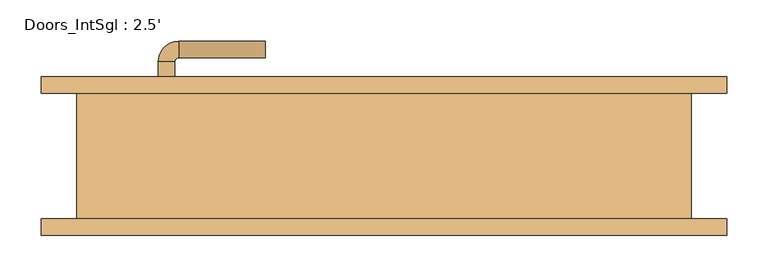
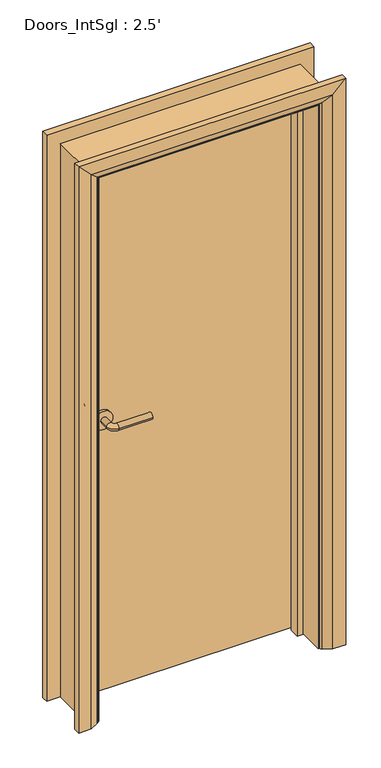
"""IFC4 building model written with IfcOpenShell, lengths in millimetres: door geometry, Doors_IntSgl : 2.5'."""

from ifc_helpers import new_model, si_unit, point, frame, frame_2d, origin, place, context, project, spatial, polyline, circle_curve, ellipse_curve, trimmed, segment, composite_curve, outline, extrude, faceted_brep, source, transform, mapped, element, save
from ifc_brep_helpers import plane_surface, cylinder_surface, revolved_surface, advanced_brep


def doors_intsgl_2_5_fba66aca(model_context):
    return source(origin(), model_context, "Body", "SolidModel", [
        advanced_brep(
        [(-274.0, 30.2, 900.0), (-254.0, 30.2, 900.0), (-254.0, 0.2, 900.0), (-274.0, 0.2, 900.0), (-249.0, -4.8, 900.0), (-249.0, -24.8, 900.0), (-144.0, -24.8, 900.0), (-144.0, -4.8, 900.0)],
        [
            (0, 1, circle_curve(frame((-264.0, 30.2, 900.0), z_axis=(0.0, 1.0, 0.0), x_axis=(1.0, 0.0, 0.0)), 10.0)),
            (1, 0, circle_curve(frame((-264.0, 30.2, 900.0), z_axis=(0.0, 1.0, 0.0), x_axis=(1.0, 0.0, 0.0)), 10.0)),
            (1, 2),
            (2, 3, circle_curve(frame((-264.0, 0.2, 900.0), z_axis=(0.0, 1.0, 0.0), x_axis=(1.0, 0.0, 0.0)), 10.0)),
            (3, 0),
            (3, 2, circle_curve(frame((-264.0, 0.2, 900.0), z_axis=(0.0, 1.0, 0.0), x_axis=(1.0, 0.0, 0.0)), 10.0)),
            (4, 5, circle_curve(frame((-249.0, -14.8, 900.0), z_axis=(-1.0, 0.0, 0.0), x_axis=(0.0, 1.0, 0.0)), 10.0)),
            (5, 3, circle_curve(frame((-249.0, 0.2, 900.0), z_axis=(0.0, 0.0, -1.0), x_axis=(-1.0, 0.0, 0.0)), 25.0)),
            (2, 4, circle_curve(frame((-249.0, 0.2, 900.0), z_axis=(0.0, 0.0, 1.0), x_axis=(-1.0, 0.0, 0.0)), 5.0)),
            (5, 4, circle_curve(frame((-249.0, -14.8, 900.0), z_axis=(-1.0, 0.0, 0.0), x_axis=(0.0, 1.0, 0.0)), 10.0)),
            (6, 7, circle_curve(frame((-144.0, -14.8, 900.0), z_axis=(1.0, 0.0, 0.0), x_axis=(0.0, 1.0, 0.0)), 10.0)),
            (7, 6, circle_curve(frame((-144.0, -14.8, 900.0), z_axis=(1.0, 0.0, 0.0), x_axis=(0.0, 1.0, 0.0)), 10.0)),
            (4, 7),
            (6, 5),
        ],
        [
            plane_surface(frame((-264.0, 30.2, 900.0), z_axis=(0.0, 1.0, 0.0), x_axis=(0.0, 0.0, 1.0))),
            cylinder_surface(frame((-264.0, 30.2, 900.0), z_axis=(0.0, 1.0, 0.0), x_axis=(1.0, 0.0, 0.0)), 10.0),
            revolved_surface(trimmed(ellipse_curve(frame((-264.0, 0.2, 900.0), z_axis=(0.0, -1.0, 0.0), x_axis=(1.0, 0.0, 0.0)), 10.0, 10.0), [point((-274.0, 0.2, 900.0))], [point((-254.0, 0.2, 900.0))], True, "CARTESIAN"), (-249.0, 0.2, 900.0), (0.0, 0.0, -1.0)),
            revolved_surface(trimmed(ellipse_curve(frame((-264.0, 0.2, 900.0), z_axis=(0.0, -1.0, 0.0), x_axis=(1.0, 0.0, 0.0)), 10.0, 10.0), [point((-254.0, 0.2, 900.0))], [point((-274.0, 0.2, 900.0))], True, "CARTESIAN"), (-249.0, 0.2, 900.0), (0.0, 0.0, -1.0)),
            plane_surface(frame((-144.0, -14.8, 900.0), z_axis=(1.0, 0.0, 0.0), x_axis=(0.0, 0.0, 1.0))),
            cylinder_surface(frame((-249.0, -14.8, 900.0), z_axis=(-1.0, 0.0, 0.0), x_axis=(0.0, 1.0, 0.0)), 10.0),
        ],
        [
            (0, [[1, 2]]),
            (1, [[3, 4, 5, -2]]),
            (1, [[-5, 6, -3, -1]]),
            (2, [[7, 8, -4, 9]]),
            (3, [[10, -9, -6, -8]]),
            (4, [[11, 12]]),
            (5, [[13, -11, 14, -7]]),
            (5, [[-14, -12, -13, -10]]),
        ],
    ),
        extrude(outline(composite_curve([segment(trimmed(circle_curve(frame_2d((900.0, -266.5)), 30.0), [point((900.0, -296.5))], [point((900.0, -236.5))], False, "CARTESIAN"), True, "CONTINUOUS"), segment(trimmed(circle_curve(frame_2d((900.0, -266.5)), 30.0), [point((900.0, -236.5))], [point((900.0, -296.5))], False, "CARTESIAN"), True, "CONTINUOUS")], self_intersect=False)), frame((0.0, 30.2, 0.0), z_axis=(0.0, 1.0, 0.0), x_axis=(0.0, 0.0, 1.0)), (0.0, 0.0, 1.0), 8.0),
        advanced_brep(
        [(-274.0, 84.2, 900.0), (-254.0, 84.2, 900.0), (-274.0, 114.2, 900.0), (-254.0, 114.2, 900.0), (-249.0, 119.2, 900.0), (-249.0, 139.2, 900.0), (-144.0, 139.2, 900.0), (-144.0, 119.2, 900.0)],
        [
            (0, 1, circle_curve(frame((-264.0, 84.2, 900.0), z_axis=(0.0, -1.0, 0.0), x_axis=(1.0, 0.0, 0.0)), 10.0)),
            (1, 0, circle_curve(frame((-264.0, 84.2, 900.0), z_axis=(0.0, -1.0, 0.0), x_axis=(1.0, 0.0, 0.0)), 10.0)),
            (0, 2),
            (2, 3, circle_curve(frame((-264.0, 114.2, 900.0), z_axis=(0.0, -1.0, 0.0), x_axis=(1.0, 0.0, 0.0)), 10.0)),
            (3, 1),
            (3, 2, circle_curve(frame((-264.0, 114.2, 900.0), z_axis=(0.0, -1.0, 0.0), x_axis=(1.0, 0.0, 0.0)), 10.0)),
            (4, 3, circle_curve(frame((-249.0, 114.2, 900.0), z_axis=(0.0, 0.0, 1.0), x_axis=(-1.0, 0.0, 0.0)), 5.0)),
            (2, 5, circle_curve(frame((-249.0, 114.2, 900.0), z_axis=(0.0, 0.0, -1.0), x_axis=(-1.0, 0.0, 0.0)), 25.0)),
            (5, 4, circle_curve(frame((-249.0, 129.2, 900.0), z_axis=(-1.0, 0.0, 0.0), x_axis=(0.0, -1.0, 0.0)), 10.0)),
            (4, 5, circle_curve(frame((-249.0, 129.2, 900.0), z_axis=(-1.0, 0.0, 0.0), x_axis=(0.0, -1.0, 0.0)), 10.0)),
            (6, 7, circle_curve(frame((-144.0, 129.2, 900.0), z_axis=(1.0, 0.0, 0.0), x_axis=(0.0, -1.0, 0.0)), 10.0)),
            (7, 6, circle_curve(frame((-144.0, 129.2, 900.0), z_axis=(1.0, 0.0, 0.0), x_axis=(0.0, -1.0, 0.0)), 10.0)),
            (5, 6),
            (7, 4),
        ],
        [
            plane_surface(frame((-264.0, 84.2, 900.0), z_axis=(0.0, -1.0, 0.0), x_axis=(0.0, 0.0, 1.0))),
            cylinder_surface(frame((-264.0, 84.2, 900.0), z_axis=(0.0, -1.0, 0.0), x_axis=(1.0, 0.0, 0.0)), 10.0),
            revolved_surface(trimmed(ellipse_curve(frame((-264.0, 114.2, 900.0), z_axis=(0.0, -1.0, 0.0), x_axis=(1.0, 0.0, 0.0)), 10.0, 10.0), [point((-274.0, 114.2, 900.0))], [point((-254.0, 114.2, 900.0))], True, "CARTESIAN"), (-249.0, 114.2, 900.0), (0.0, 0.0, -1.0)),
            revolved_surface(trimmed(ellipse_curve(frame((-264.0, 114.2, 900.0), z_axis=(0.0, -1.0, 0.0), x_axis=(1.0, 0.0, 0.0)), 10.0, 10.0), [point((-254.0, 114.2, 900.0))], [point((-274.0, 114.2, 900.0))], True, "CARTESIAN"), (-249.0, 114.2, 900.0), (0.0, 0.0, -1.0)),
            plane_surface(frame((-144.0, 129.2, 900.0), z_axis=(1.0, 0.0, 0.0), x_axis=(0.0, 0.0, 1.0))),
            cylinder_surface(frame((-249.0, 129.2, 900.0), z_axis=(-1.0, 0.0, 0.0), x_axis=(0.0, -1.0, 0.0)), 10.0),
        ],
        [
            (0, [[1, 2]]),
            (1, [[-1, 3, 4, 5]]),
            (1, [[-2, -5, 6, -3]]),
            (2, [[7, -4, 8, 9]]),
            (3, [[-8, -6, -7, 10]]),
            (4, [[11, 12]]),
            (5, [[-9, 13, -12, 14]]),
            (5, [[-10, -14, -11, -13]]),
        ],
    ),
        extrude(outline(composite_curve([segment(trimmed(circle_curve(frame_2d((900.0, -266.5)), 30.0), [point((900.0, -296.5))], [point((900.0, -236.5))], False, "CARTESIAN"), True, "CONTINUOUS"), segment(trimmed(circle_curve(frame_2d((900.0, -266.5)), 30.0), [point((900.0, -236.5))], [point((900.0, -296.5))], False, "CARTESIAN"), True, "CONTINUOUS")], self_intersect=False)), frame((0.0, 76.2, 0.0), z_axis=(0.0, 1.0, 0.0), x_axis=(0.0, 0.0, 1.0)), (0.0, 0.0, 1.0), 8.0),
        extrude(outline(polyline([(339.0, 38.2), (-339.0, 38.2), (-339.0, 76.2), (339.0, 76.2), (339.0, 38.2)])), frame((0.0, 0.0, 8.0), z_axis=(0.0, 0.0, 1.0), x_axis=(1.0, 0.0, 0.0)), (0.0, 0.0, 1.0), 1778.8),
        advanced_brep(
        [(416.0, 96.2, 0.0), (416.0, 76.2, 0.0), (346.0, 76.2, 0.0), (350.0, 82.2, 0.0), (376.0, 96.2, 0.0), (416.0, 96.2, 1863.8), (416.0, 76.2, 1863.8), (-416.0, 76.2, 1863.8), (-416.0, 76.2, 0.0), (-346.0, 76.2, 0.0), (-346.0, 76.2, 1793.8), (346.0, 76.2, 1793.8), (350.0, 82.2, 1797.8), (376.0, 96.2, 1823.8), (-376.0, 96.2, 1823.8), (-376.0, 96.2, 0.0), (-416.0, 96.2, 0.0), (-416.0, 96.2, 1863.8), (-350.0, 82.2, 0.0), (-350.0, 82.2, 1797.8)],
        [
            (0, 1),
            (1, 2),
            (2, 3, circle_curve(frame((354.0, 75.2, 0.0), z_axis=(0.0, 0.0, -1.0), x_axis=(1.0, 0.0, 0.0)), 8.0622577)),
            (3, 4),
            (4, 0),
            (0, 5),
            (5, 6),
            (6, 1),
            (6, 7),
            (7, 8),
            (8, 9),
            (9, 10),
            (10, 11),
            (11, 2),
            (11, 12, ellipse_curve(frame((354.0, 75.2, 1801.8), z_axis=(0.7071067811865475, 0.0, -0.7071067811865475), x_axis=(-0.7071067811865474, 0.0, -0.7071067811865476)), 11.4017543, 8.0622577)),
            (12, 3),
            (12, 13),
            (13, 4),
            (13, 14),
            (14, 15),
            (15, 16),
            (16, 17),
            (17, 5),
            (7, 17),
            (16, 8),
            (15, 18),
            (18, 9, circle_curve(frame((-354.0, 75.2, 0.0), z_axis=(0.0, 0.0, -1.0), x_axis=(-1.0, 0.0, 0.0)), 8.0622577)),
            (19, 10, ellipse_curve(frame((-354.0, 75.2, 1801.8), z_axis=(-0.7071067811865475, 0.0, -0.7071067811865475), x_axis=(-0.7071067811865474, 0.0, 0.7071067811865476)), 11.4017543, 8.0622577)),
            (18, 19),
            (14, 19),
            (19, 12),
        ],
        [
            plane_surface(frame((346.0, 76.2, 0.0), z_axis=(0.0, 0.0, -1.0), x_axis=(0.0, -1.0, 0.0))),
            plane_surface(frame((416.0, 96.2, 0.0), z_axis=(1.0, 0.0, 0.0), x_axis=(0.0, 0.0, 1.0))),
            plane_surface(frame((416.0, 76.2, 0.0), z_axis=(0.0, -1.0, 0.0), x_axis=(0.0, 0.0, 1.0))),
            cylinder_surface(frame((354.0, 75.2, 0.0), z_axis=(0.0, 0.0, -1.0), x_axis=(1.0, 0.0, 0.0)), 8.0622577),
            plane_surface(frame((350.0, 82.2, 0.0), z_axis=(-0.4740998230350126, 0.880471099922178, 0.0), x_axis=(0.0, 0.0, 1.0))),
            plane_surface(frame((376.0, 96.2, 0.0), z_axis=(0.0, 1.0, 0.0), x_axis=(0.0, 0.0, 1.0))),
            plane_surface(frame((-416.0, 96.2, 1863.8), z_axis=(-1.0, 0.0, 0.0), x_axis=(0.0, 0.0, -1.0))),
            plane_surface(frame((-346.0, 76.2, 0.0), z_axis=(0.0, 0.0, -1.0), x_axis=(0.0, -1.0, 0.0))),
            cylinder_surface(frame((-354.0, 75.2, 1793.8), z_axis=(0.0, 0.0, 1.0), x_axis=(-1.0, 0.0, 0.0)), 8.0622577),
            plane_surface(frame((-350.0, 82.2, 1797.8), z_axis=(0.47409982303501824, 0.8804710999221749, 0.0), x_axis=(0.0, 0.0, -1.0))),
            plane_surface(frame((416.0, 96.2, 1863.8), z_axis=(0.0, 0.0, 1.0), x_axis=(-1.0, 0.0, 0.0))),
            cylinder_surface(frame((346.0, 75.2, 1801.8), z_axis=(1.0, 0.0, 0.0), x_axis=(0.0, 0.0, 1.0)), 8.0622577),
            plane_surface(frame((350.0, 82.2, 1797.8), z_axis=(0.0, 0.8804710999221764, -0.4740998230350154), x_axis=(-1.0, 0.0, 0.0))),
        ],
        [
            (0, [[1, 2, 3, 4, 5]]),
            (1, [[-1, 6, 7, 8]]),
            (2, [[-2, -8, 9, 10, 11, 12, 13, 14]]),
            (3, [[-3, -14, 15, 16]]),
            (4, [[-4, -16, 17, 18]]),
            (5, [[-5, -18, 19, 20, 21, 22, 23, -6]]),
            (6, [[24, -22, 25, -10]]),
            (7, [[-21, 26, 27, -11, -25]]),
            (8, [[28, -12, -27, 29]]),
            (9, [[30, -29, -26, -20]]),
            (10, [[-7, -23, -24, -9]]),
            (11, [[-15, -13, -28, 31]]),
            (12, [[-17, -31, -30, -19]]),
        ],
    ),
        extrude(outline(polyline([(0.0, -341.0), (0.0, -322.0), (1769.8, -322.0), (1769.8, 322.0), (0.0, 322.0), (0.0, 341.0), (1788.8, 341.0), (1788.8, -341.0), (0.0, -341.0)])), frame((0.0, 4.2, 0.0), z_axis=(0.0, 1.0, 0.0), x_axis=(0.0, 0.0, 1.0)), (0.0, 0.0, 1.0), 32.0),
        advanced_brep(
        [(-416.0, -96.2, 0.0), (-416.0, -76.2, 0.0), (-346.0, -76.2, 0.0), (-350.0, -82.2, 0.0), (-376.0, -96.2, 0.0), (-416.0, -96.2, 1863.8), (-416.0, -76.2, 1863.8), (-346.0, -76.2, 1793.8), (-350.0, -82.2, 1797.8), (-376.0, -96.2, 1823.8), (416.0, -96.2, 0.0), (376.0, -96.2, 0.0), (350.0, -82.2, 0.0), (346.0, -76.2, 0.0), (416.0, -76.2, 0.0), (416.0, -96.2, 1863.8), (376.0, -96.2, 1823.8), (350.0, -82.2, 1797.8), (346.0, -76.2, 1793.8), (416.0, -76.2, 1863.8)],
        [
            (0, 1),
            (1, 2),
            (2, 3, circle_curve(frame((-354.0, -75.2, 0.0), z_axis=(0.0, 0.0, -1.0), x_axis=(-1.0, 0.0, 0.0)), 8.0622577)),
            (3, 4),
            (4, 0),
            (0, 5),
            (5, 6),
            (6, 1),
            (6, 7),
            (7, 2),
            (7, 8, ellipse_curve(frame((-354.0, -75.2, 1801.8), z_axis=(-0.7071067811865475, 0.0, -0.7071067811865475), x_axis=(0.7071067811865474, 0.0, -0.7071067811865476)), 11.4017543, 8.0622577)),
            (8, 3),
            (8, 9),
            (9, 4),
            (9, 5),
            (10, 11),
            (11, 12),
            (12, 13, circle_curve(frame((354.0, -75.2, 0.0), z_axis=(0.0, 0.0, -1.0), x_axis=(1.0, 0.0, 0.0)), 8.0622577)),
            (13, 14),
            (14, 10),
            (15, 16),
            (16, 11),
            (10, 15),
            (16, 17),
            (17, 12),
            (17, 18, ellipse_curve(frame((354.0, -75.2, 1801.8), z_axis=(0.7071067811865475, 0.0, -0.7071067811865475), x_axis=(0.7071067811865474, 0.0, 0.7071067811865476)), 11.4017543, 8.0622577)),
            (18, 13),
            (18, 19),
            (19, 14),
            (19, 15),
            (5, 15),
            (19, 6),
            (18, 7),
            (17, 8),
            (16, 9),
        ],
        [
            plane_surface(frame((-346.0, -149.0010989, 0.0), z_axis=(0.0, 0.0, -1.0), x_axis=(1.0, 0.0, 0.0))),
            plane_surface(frame((-416.0, -96.2, 0.0), z_axis=(-1.0, 0.0, 0.0), x_axis=(0.0, 0.0, 1.0))),
            plane_surface(frame((-416.0, -76.2, 0.0), z_axis=(0.0, 1.0, 0.0), x_axis=(0.0, 0.0, 1.0))),
            cylinder_surface(frame((-354.0, -75.2, 0.0), z_axis=(0.0, 0.0, -1.0), x_axis=(-1.0, 0.0, 0.0)), 8.0622577),
            plane_surface(frame((-350.0, -82.2, 0.0), z_axis=(0.4740998230350183, -0.8804710999221749, 0.0), x_axis=(0.0, 0.0, 1.0))),
            plane_surface(frame((-376.0, -96.2, 0.0), z_axis=(0.0, -1.0, 0.0), x_axis=(0.0, 0.0, 1.0))),
            plane_surface(frame((346.0, -149.0010989, 0.0), z_axis=(0.0, 0.0, -1.0), x_axis=(-1.0, 0.0, 0.0))),
            plane_surface(frame((376.0, -96.2, 1823.8), z_axis=(0.0, -1.0, 0.0), x_axis=(0.0, 0.0, -1.0))),
            plane_surface(frame((350.0, -82.2, 1797.8), z_axis=(-0.4740998230350183, -0.8804710999221749, 0.0), x_axis=(0.0, 0.0, -1.0))),
            cylinder_surface(frame((354.0, -75.2, 1793.8), z_axis=(0.0, 0.0, 1.0), x_axis=(1.0, 0.0, 0.0)), 8.0622577),
            plane_surface(frame((416.0, -76.2, 1863.8), z_axis=(0.0, 1.0, 0.0), x_axis=(0.0, 0.0, -1.0))),
            plane_surface(frame((416.0, -96.2, 1863.8), z_axis=(1.0, 0.0, 0.0), x_axis=(0.0, 0.0, -1.0))),
            plane_surface(frame((-416.0, -96.2, 1863.8), z_axis=(0.0, 0.0, 1.0), x_axis=(1.0, 0.0, 0.0))),
            plane_surface(frame((-416.0, -76.2, 1863.8), z_axis=(0.0, 1.0, 0.0), x_axis=(1.0, 0.0, 0.0))),
            cylinder_surface(frame((-346.0, -75.2, 1801.8), z_axis=(-1.0, 0.0, 0.0), x_axis=(0.0, 0.0, 1.0)), 8.0622577),
            plane_surface(frame((-350.0, -82.2, 1797.8), z_axis=(0.0, -0.8804710999221749, -0.4740998230350183), x_axis=(1.0, 0.0, 0.0))),
            plane_surface(frame((-376.0, -96.2, 1823.8), z_axis=(0.0, -1.0, 0.0), x_axis=(1.0, 0.0, 0.0))),
        ],
        [
            (0, [[1, 2, 3, 4, 5]]),
            (1, [[-1, 6, 7, 8]]),
            (2, [[-2, -8, 9, 10]]),
            (3, [[-3, -10, 11, 12]]),
            (4, [[-4, -12, 13, 14]]),
            (5, [[-5, -14, 15, -6]]),
            (6, [[16, 17, 18, 19, 20]]),
            (7, [[21, 22, -16, 23]]),
            (8, [[24, 25, -17, -22]]),
            (9, [[26, 27, -18, -25]]),
            (10, [[28, 29, -19, -27]]),
            (11, [[30, -23, -20, -29]]),
            (12, [[-7, 31, -30, 32]]),
            (13, [[-9, -32, -28, 33]]),
            (14, [[-11, -33, -26, 34]]),
            (15, [[-13, -34, -24, 35]]),
            (16, [[-15, -35, -21, -31]]),
        ],
    ),
        faceted_brep([(-341.0, 76.2, 0.0), (-341.0, -76.2, 0.0), (-373.0, -76.2, 0.0), (-373.0, 76.2, 0.0), (-341.0, 76.2, 1788.8), (-341.0, -76.2, 1788.8), (-373.0, -76.2, 1820.8), (-373.0, 76.2, 1820.8), (341.0, 76.2, 0.0), (373.0, 76.2, 0.0), (373.0, -76.2, 0.0), (341.0, -76.2, 0.0), (341.0, 76.2, 1788.8), (373.0, 76.2, 1820.8), (373.0, -76.2, 1820.8), (341.0, -76.2, 1788.8)], [[[0, 1, 2, 3]], [[1, 0, 4, 5]], [[2, 1, 5, 6]], [[3, 2, 6, 7]], [[0, 3, 7, 4]], [[8, 9, 10, 11]], [[12, 13, 9, 8]], [[13, 14, 10, 9]], [[14, 15, 11, 10]], [[15, 12, 8, 11]], [[5, 4, 12, 15]], [[6, 5, 15, 14]], [[7, 6, 14, 13]], [[4, 7, 13, 12]]]),
    ])


if __name__ == "__main__":
    model = new_model("IFC4")
    model_context = context("Model", 3, world=origin())
    ifc_project = project(units=[si_unit("LENGTHUNIT", "METRE", prefix="MILLI")], contexts=[model_context])
    site = spatial("IfcSite", under=ifc_project)
    building = spatial("IfcBuilding", under=site)
    placement = place(None, origin())
    doors_intsgl_2_5_shape = doors_intsgl_2_5_fba66aca(model_context)
    element("IfcDoor", 1, ObjectType="Doors_IntSgl : 2.5'", at=placement, inside=building, context=model_context, shape_type="MappedRepresentation", body=[
        mapped(doors_intsgl_2_5_shape, transform((0.0, 0.0, 0.0), x_axis=(1.0, 0.0, 0.0), y_axis=(0.0, 1.0, 0.0), z_axis=(0.0, 0.0, 1.0))),
    ])
    save(model, "model.ifc")

# Revit data of these elements
# Type "Doors_IntSgl : 2.5'"
#   Type Mark = "49"
#   Type Comments = "Internal Single"
#   Operation = "SingleSwingRight"
#   Manufacturer = "Revit"
#   Keynote = "L20"
#   Description = "Internal Single Door"
#   Analytic Construction = "Metal"
#   UnderCut = 0' - 0.31496"
#   Tolerance = 0' - 0.07874"
#   Thickness = 0' - 1.49606"
#   Thermal Resistance (R) = 0.270117 (m²·K)/W
#   Structural Tolerance = 0' - 0.31496"
#   StopDepth = 0' - 1.25984"
#   Stop Thickness = 0' - 0.74803"
#   Rough Width = 2' - 6"
#   Rough Height = 6' - 0"
#   Height to Top Lock Rail = 3' - 3.37008"
#   Heat Transfer Coefficient (U) = 3.7021 W/(m²·K)
#   Handle Z Distance = 2' - 11.43307"
#   Handle X Distance = 0' - 2.95276"
#   Frame Thickness = 0' - 1.25984"
#   Door Panel Width = 2' - 2.69291"
#   Door Panel Thickness = 0' - 1.49606"
#   Door Panel Offset = 0' - 0"
#   Height = 6' - 0"
#   Width = 2' - 6"
#   Door Panel Height = 5' - 10.0315"
#   Architrave Setback = 0' - 0.19685"
#   Vis - Ironmongery = yes
#   Material Ironmongery = Door - Handle
#   Material Frame = Door - Frame/Mullion (1)
#   Material Door = Door - Panel
#   Material Architrave = Door - Architrave
#   Visual Light Transmittance = 0
#   Solar Heat Gain Coefficient = 0
#   Function = (empty or 0)
#   Wall Closure = (empty or 0)
# Element 1 (IfcDoor, "Doors_IntSgl : 2.5'")
#   Materials on its faces: "Door - Architrave", "Door - Handle", "Door - Frame/Mullion (1)", "Door - Panel"
# Materials
#   "Door - Handle": colour RGB 0 0 0, transparency 0, Keynote = "P21", Cost = 0
#   "Door - Frame/Mullion (1)": class "Wood", colour RGB 212 179 113, transparency 0, Keynote = "L20", Cost = 0
#   "Door - Panel": class "Wood", colour RGB 210 159 95, transparency 0, Keynote = "L20", Cost = 0
#   "Door - Architrave": class "Wood", colour RGB 154 90 5, transparency 0, Keynote = "P20", Cost = 0
